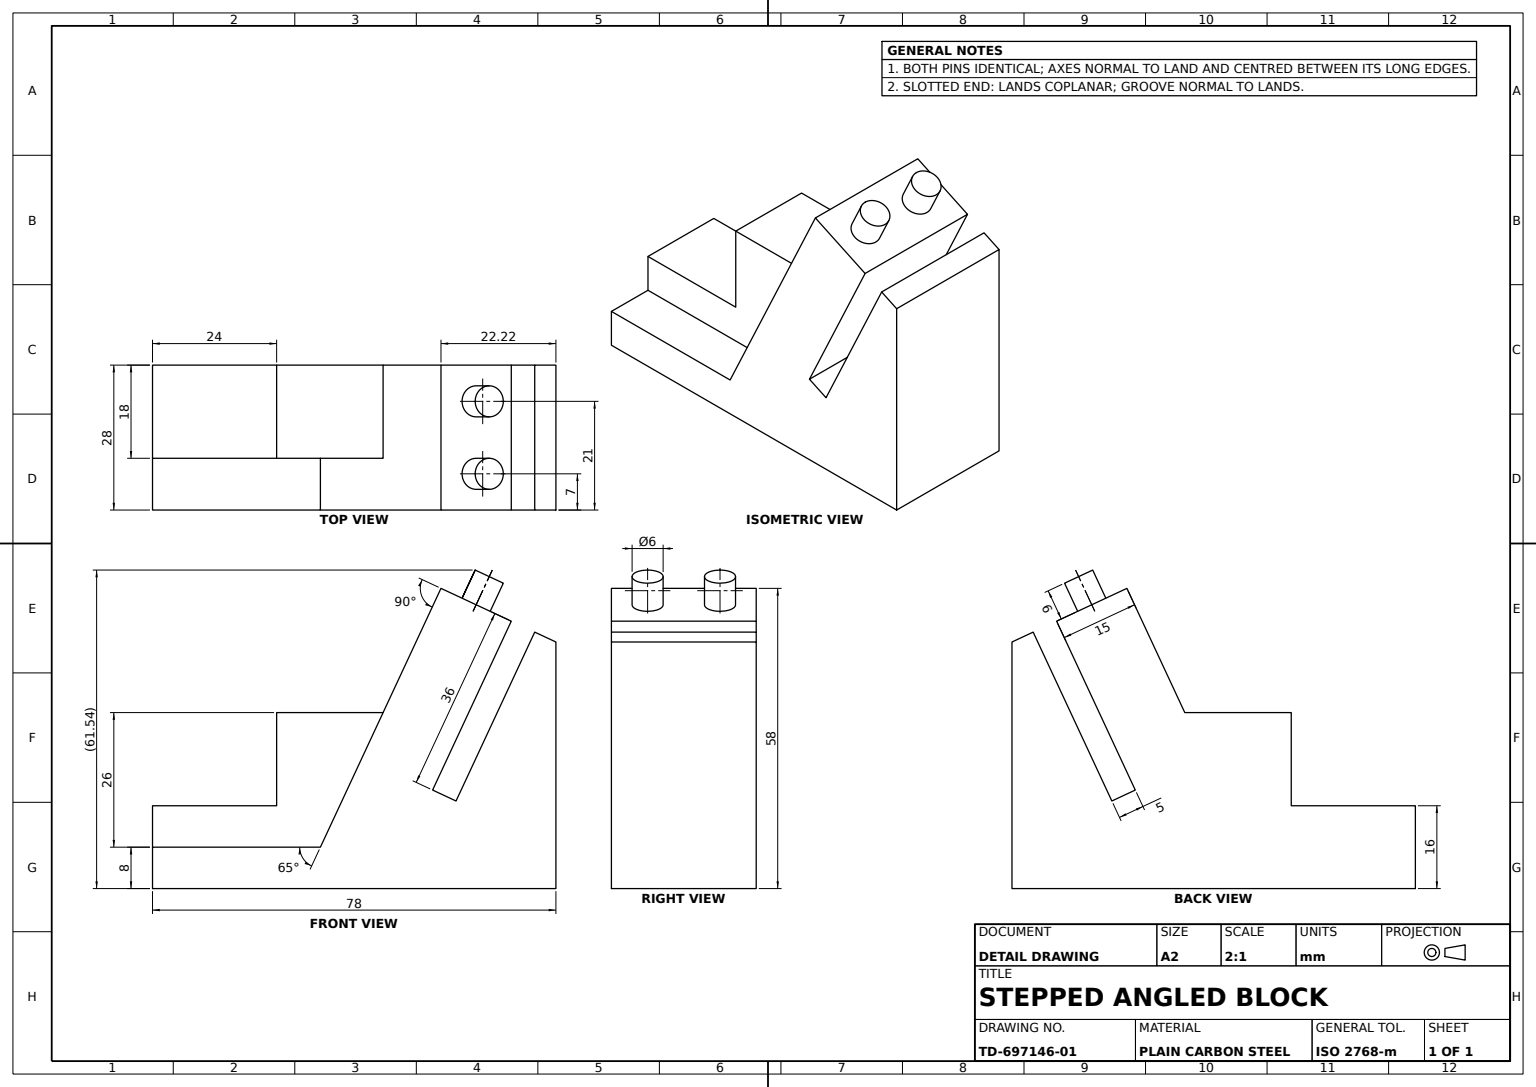
SolidWorks part; units mm, degrees
material "Plain Carbon Steel"
ref_plane "Front Plane" through (0, 0, 0) normal (0, 0, 1) x (1, 0, 0)
ref_plane "Top Plane" through (0, 0, 0) normal (0, 1, 0) x (1, 0, 0)
ref_plane "Right Plane" through (0, 0, 0) normal (1, 0, 0) x (0, 0, -1)
sketch "Base Profile Sketch" plane through (0, 0, 0) normal (0, 0, 1) x (1, 0, 0)
  line L0 (0, 0) -> (0, 8)
  line L1 (0, 8) -> (32.4615, 8)
  line L2 (32.4615, 8) -> (55.7769, 58)
  line L3 (55.7769, 58) -> (69.3715, 51.6607)
  line L4 (69.3715, 51.6607) -> (54.1573, 19.0336)
  line L5 (54.1573, 19.0336) -> (58.6888, 16.9206)
  line L6 (58.6888, 16.9206) -> (73.9031, 49.5476)
  line L8 (78, 47.6372) -> (78, 0)
  line L9 (78, 0) -> (0, 0)
  line L10 (73.9031, 49.5476) -> (78, 47.6372)
  dimension "D1" = 78
  dimension "D2" = 8
  dimension "D3" = 65
  dimension "D4" = 36
  dimension "D5" = 58
  dimension "D6" = 5
  dimension "D7" = 24.5205
  dimension "D8" = 15
extrude "Stepped Base Block" add sketch "Base Profile Sketch" along normal blind 28
ref_plane "Plane1" through (0, 0, 0) normal (0, 0, 1) x (1, 0, 0)
sketch "Riser Block Sketch" plane through (0, 0, 0) normal (-1, 0, 0) x (0, 0, 1)
  line L0 (0, 0) -> (18, 0)
  line L1 (28, 0) -> (0, 0) construction
  line L2 (18, 0) -> (18, 16)
  line L3 (18, 16) -> (0, 16)
  line L4 (0, -33.8448) -> (0, 33.8448) construction
  line L5 (0, 16) -> (0, 0)
  dimension "D1" = 16
  dimension "D2" = 18
extrude "Riser Block 16x18" add sketch "Riser Block Sketch" against normal up to next
extrude "Locating Pins x2" add sketch "Locating Pins Sketch" along normal blind 6
sketch "Locating Pins Sketch" plane through (32.1774, 69.0046, 0) normal (0.4226, 0.9063, 0) x (0.9063, -0.4226, 0)
  line L2 (-33.8448, 0) -> (33.8448, 0) construction
  circle A0 centre (33.5392, -7) radius 3
  circle A1 centre (33.5392, -21) radius 3
  dimension "D1" = 6
  dimension "D2" = 6
  dimension "D3" = 7.5
  dimension "D4" = 7
  dimension "D5" = 21
ref_plane "Plane6" through (24, 0, 0) normal (-1, 0, 0) x (0, 0, 1)
ref_plane "Plane2" through (24, 0, 0) normal (-1, 0, 0) x (0, 0, 1)
sketch "Angled Head Sketch" plane through (24, 0, 0) normal (-1, 0, 0) x (0, 0, 1)
  line L0 (18, 16) -> (0, 16)
  line L1 (18, 16) -> (18, 34)
  line L2 (0, 16) -> (0, 34)
  line L3 (18, 34) -> (0, 34)
  line L4 (0, -33.8448) -> (0, 33.8448) construction
  line L5 (18, 16) -> (0, 16) construction
  dimension "D1" = 18
extrude "Angled Head Block" add sketch "Angled Head Sketch" against normal blind 26
